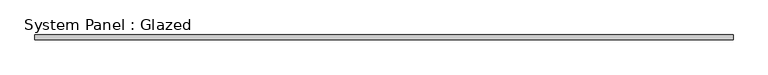
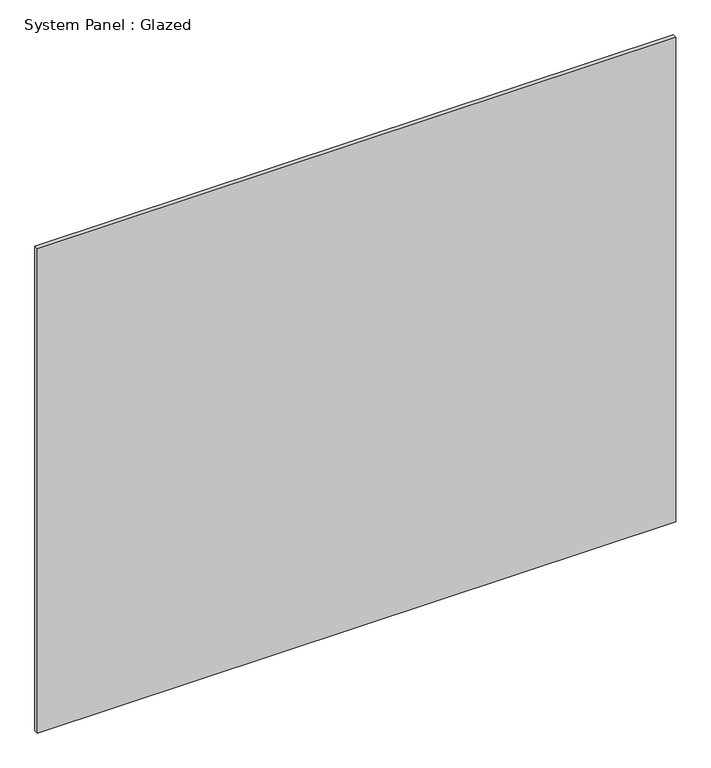
"""IFC4 building model written with IfcOpenShell, lengths in millimetres: plate geometry, System Panel : Glazed."""

from ifc_helpers import new_model, si_unit, origin, origin_with_axes, place, context, project, spatial, polyline, outline, extrude, source, transform, mapped, element, save


def system_panel_glazed_dc472efa(model_context):
    return source(origin(), model_context, "Body", "SweptSolid", [
        extrude(outline(polyline([(1821.0241767, 19.05), (-1821.0241767, 19.05), (-1821.0241767, 44.45), (1821.0241767, 44.45), (1821.0241767, 19.05)])), origin_with_axes(), (0.0, 0.0, 1.0), 2921.0),
    ])


if __name__ == "__main__":
    model = new_model("IFC4")
    model_context = context("Model", 3, world=origin())
    ifc_project = project(units=[si_unit("LENGTHUNIT", "METRE", prefix="MILLI")], contexts=[model_context])
    site = spatial("IfcSite", under=ifc_project)
    building = spatial("IfcBuilding", under=site)
    placement = place(None, origin())
    system_panel_glazed_shape = system_panel_glazed_dc472efa(model_context)
    element("IfcPlate", 1, ObjectType="System Panel : Glazed", at=placement, inside=building, context=model_context, shape_type="MappedRepresentation", body=[
        mapped(system_panel_glazed_shape, transform((0.0, 0.0, 0.0), x_axis=(1.0, 0.0, 0.0), y_axis=(0.0, 1.0, 0.0), z_axis=(0.0, 0.0, 1.0))),
    ])
    save(model, "model.ifc")

# Revit data of these elements
# Type "System Panel : Glazed"
#   Construction Type Id = "GSP4R"
#   Analytic Construction = "1/8 in Pilkington single glazing"
#   Visual Light Transmittance = 0.9
#   Solar Heat Gain Coefficient = 0.86
#   Heat Transfer Coefficient (U) = 1.18115 BTU/(h·ft²·°F)
#   Define Thermal Properties by = 1
# Element 1 (IfcPlate, "System Panel : Glazed")
#   Materials on its faces: "Glass"
# Materials
#   "Glass": class "Glass", colour RGB 0 128 192, transparency 0.75, Description = "Soda Lime Glass", Cost = 0
